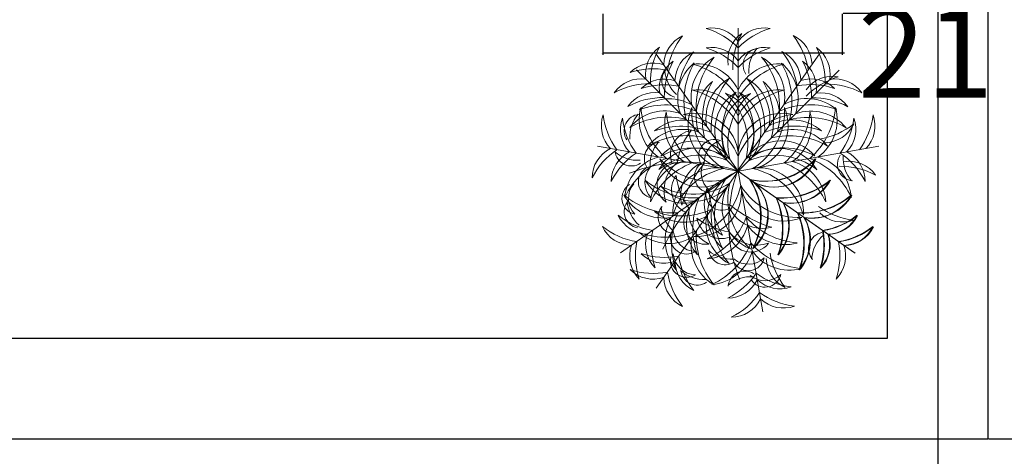
# Model space of a CAD drawing. Units: inches. Extents: x -48 to 50072, y 0 to 21068.
# Tile 33 of 75: x 467 to 555, y 213 to 251. Entities that reach past the tile are written whole.
import ezdxf

# ---------------------------------------------------------------- set-up
doc = ezdxf.new("R2010")
doc.units = ezdxf.units.IN
doc.header["$MEASUREMENT"] = 0
doc.linetypes.add('ACAD_ISO02W100', pattern=[15, 12, -3])
for name, color, linetype, lineweight in [('A-ANNO-DIMS', 2, 'Continuous', 18), ('C-PROP', 7, 'Continuous', 25), ('C-PROP-REF', 32, 'ACAD_ISO02W100', 13), ('L-PLNT', 94, 'Continuous', 13)]:
    doc.layers.add(name, color=color, linetype=linetype, lineweight=lineweight)
doc.styles.get("Standard").update_dxf_attribs({"font": 'arial.ttf'})
doc.dimstyles.get("Standard").update_dxf_attribs({"dimtxt": 8, "dimasz": 0.18, "dimexe": 0.18, "dimexo": 0.0625, "dimgap": 0.09, "dimtad": 0, "dimtih": 1, "dimtoh": 1, "dimdec": 1, "dimzin": 0, "dimdsep": 46, "dimlunit": 4, "dimtxsty": 'Standard', "dimblk": 'ARCHTICK', "dimcen": 0.09, "dimadec": 0, "dimazin": 0, "dimtfac": 1, "dimtdec": 1, "dimtofl": 0, "dimtmove": 0, "dimatfit": 3, "dimldrblk": 'ARCHTICK', "dimfxl": 1, "dimtolj": 1, "dimtzin": 0, "dimarcsym": 0})

# ---------------------------------------------------------------- blocks, each defined once
blk = doc.blocks.new('A$C5D061C3B')
for p, q in [((3.377, 6.679), (3.377, 3.377)), ((1.483, 6.082), (3.377, 3.377)), ((5.259, 6.086), (3.365, 3.381)), ((1.03, 5.716), (3.365, 3.381)), ((5.712, 5.712), (3.377, 3.377)), ((0.125, 3.951), (3.377, 3.377)), ((6.629, 3.951), (3.377, 3.377)), ((0.66, 1.487), (3.365, 3.381)), ((1.483, 0.672), (3.377, 3.377)), ((6.07, 1.487), (3.365, 3.381)), ((3.951, 0.125), (3.377, 3.377)), ((6.082, 1.483), (3.377, 3.377))]:
    blk.add_line(p, q)
for centre, radius, start, end in [((2.763, 5.924), 0.762, 36.29, 99.6243), ((2.145, 5.032), 1.715, 44.0763, 73.3794), ((3.991, 5.924), 0.762, 80.3757, 143.71), ((4.61, 5.032), 1.715, 106.6206, 135.9237), ((2.419, 5.816), 0.762, 115.3757, 178.71), ((3.438, 5.44), 1.715, 141.6206, 170.9237), ((3.901, 5.939), 0.762, 125.3757, 188.71), ((4.969, 5.745), 1.715, 151.6206, 180.9237), ((3.305, 5.444), 1.715, 9.0763, 38.3794), ((4.323, 5.82), 0.762, 1.29, 64.6243), ((1.998, 5.617), 0.762, 125.3757, 188.71), ((3.066, 5.423), 1.715, 151.6206, 180.9237), ((2.763, 5.474), 0.762, 36.29, 99.6243), ((2.145, 4.581), 1.715, 44.0763, 73.3794), ((3.991, 5.474), 0.762, 80.3757, 143.71), ((4.61, 4.581), 1.715, 106.6206, 135.9237), ((3.871, 5.832), 0.38, 94.742, 213.7475), ((4.447, 5.681), 0.826, 139.618, 183.2106), ((4.744, 5.613), 0.762, 351.29, 54.6243), ((3.676, 5.419), 1.715, 359.0763, 28.3794), ((2.317, 5.298), 0.762, 125.3757, 188.71), ((3.385, 5.104), 1.715, 151.6206, 180.9237), ((2.678, 5.447), 0.762, 115.3757, 178.71), ((3.696, 5.07), 1.715, 141.6206, 170.9237), ((3.344, 5.089), 1.056, 119.6063, 189.7511), ((4.177, 4.869), 1.77, 139.9634, 183.6288), ((3.398, 5.094), 1.056, 350.2489, 60.3937), ((2.565, 4.873), 1.77, 356.3712, 40.0366), ((4.064, 5.451), 0.762, 1.29, 64.6243), ((3.046, 5.075), 1.715, 9.0763, 38.3794), ((1.413, 5.111), 0.762, 71.29, 134.6243), ((1.419, 4.026), 1.715, 79.0763, 108.3794), ((1.991, 5.462), 0.38, 139.742, 258.7475), ((2.505, 5.763), 0.826, 184.618, 228.2106), ((3.035, 5.062), 1.056, 129.6063, 199.7511), ((3.894, 4.989), 1.77, 149.9634, 193.6288), ((2.422, 4.799), 1.056, 25.2489, 95.3937), ((1.866, 4.14), 1.77, 31.3712, 75.0366), ((4.332, 4.799), 1.056, 84.6063, 154.7511), ((4.888, 4.14), 1.77, 104.9634, 148.6288), ((2.848, 4.985), 1.77, 346.3712, 30.0366), ((3.707, 5.058), 1.056, 340.2489, 50.3937), ((3.357, 5.1), 1.715, 359.0763, 28.3794), ((4.425, 5.294), 0.762, 351.29, 54.6243), ((1.13, 4.748), 0.762, 81.29, 144.6243), ((1.671, 4.742), 0.762, 71.29, 134.6243), ((3.688, 4.597), 1.056, 119.6063, 189.7511), ((4.522, 4.377), 1.77, 139.9634, 183.6288), ((2.221, 4.381), 1.77, 356.3712, 40.0366), ((3.054, 4.602), 1.056, 350.2489, 60.3937), ((5.071, 4.746), 0.762, 45.3757, 108.71), ((5.564, 4.807), 0.762, 80.3757, 143.71), ((6.182, 3.914), 1.715, 106.6206, 135.9237), ((5.613, 4.744), 0.762, 35.3757, 98.71), ((1.324, 3.68), 1.715, 89.0763, 118.3794), ((1.677, 3.657), 1.715, 79.0763, 108.3794), ((2.422, 4.198), 1.056, 25.2489, 95.3937), ((1.866, 3.54), 1.77, 31.3712, 75.0366), ((3.46, 4.637), 1.056, 129.6063, 199.7511), ((4.319, 4.565), 1.77, 149.9634, 193.6288), ((4.332, 4.198), 1.056, 84.6063, 154.7511), ((4.888, 3.54), 1.77, 104.9634, 148.6288), ((3.283, 4.633), 1.056, 340.2489, 50.3937), ((2.424, 4.56), 1.77, 346.3712, 30.0366), ((5.065, 3.661), 1.715, 71.6206, 100.9237), ((5.419, 3.676), 1.715, 61.6206, 90.9237), ((1.448, 4.43), 0.762, 81.29, 144.6243), ((1.642, 3.362), 1.715, 89.0763, 118.3794), ((1.78, 3.994), 1.056, 60.2489, 130.3937), ((3.868, 4.321), 1.029, 121.3654, 221.5741), ((4.556, 4.237), 1.557, 141.8122, 203.3335), ((4.035, 4.215), 1.029, 111.3654, 211.5741), ((2.707, 4.219), 1.029, 328.4259, 68.6346), ((2.044, 4.017), 1.557, 346.6665, 48.1878), ((4.698, 4.013), 1.557, 131.8122, 193.3335), ((2.187, 4.233), 1.557, 336.6665, 38.1878), ((2.875, 4.316), 1.029, 318.4259, 58.6346), ((4.963, 3.998), 1.056, 49.6063, 119.7511), ((5.1, 3.357), 1.715, 61.6206, 90.9237), ((5.294, 4.425), 0.762, 35.3757, 98.71), ((2.143, 4.564), 1.056, 164.6063, 234.7511), ((1.702, 3.136), 1.77, 66.3712, 110.0366), ((2.888, 4.998), 1.77, 184.9634, 228.6288), ((3.25, 4.435), 1.029, 156.3654, 256.5741), ((3.862, 4.761), 1.557, 176.8122, 238.3335), ((2.893, 4.761), 1.557, 301.6665, 3.1878), ((3.504, 4.435), 1.029, 283.4259, 23.6346), ((5.04, 3.14), 1.77, 69.9634, 113.6288), ((3.866, 4.998), 1.77, 311.3712, 355.0366), ((4.611, 4.564), 1.056, 305.2489, 15.3937), ((0.975, 4.424), 0.762, 160.3757, 223.71), ((1.962, 4.878), 1.715, 186.6206, 215.9237), ((1.419, 4.346), 0.762, 160.3757, 223.71), ((2.405, 4.8), 1.715, 186.6206, 215.9237), ((1.12, 4.31), 0.38, 94.742, 213.7475), ((1.696, 4.159), 0.826, 139.618, 183.2106), ((1.685, 3.712), 1.056, 70.2489, 140.3937), ((1.757, 2.853), 1.77, 76.3712, 120.0366), ((2.124, 3.502), 1.056, 60.2489, 130.3937), ((2.734, 4.46), 1.056, 164.6063, 234.7511), ((3.48, 4.893), 1.77, 184.9634, 228.6288), ((2.358, 3.686), 1.029, 3.4259, 103.6346), ((1.93, 3.14), 1.557, 21.6665, 83.1878), ((4.397, 3.686), 1.029, 76.3654, 176.5741), ((4.824, 3.14), 1.557, 96.8122, 158.3335), ((4.618, 3.506), 1.056, 49.6063, 119.7511), ((3.275, 4.893), 1.77, 311.3712, 355.0366), ((4.985, 2.848), 1.77, 59.9634, 103.6288), ((4.02, 4.46), 1.056, 305.2489, 15.3937), ((5.058, 3.707), 1.056, 39.6063, 109.7511), ((4.349, 4.8), 1.715, 324.0763, 353.3794), ((5.335, 4.346), 0.762, 316.29, 19.6243), ((4.793, 4.878), 1.715, 324.0763, 353.3794), ((5.779, 4.424), 0.762, 316.29, 19.6243), ((2.109, 3.287), 1.056, 70.2489, 140.3937), ((2.046, 2.644), 1.77, 66.3712, 110.0366), ((4.696, 2.648), 1.77, 69.9634, 113.6288), ((4.633, 3.283), 1.056, 39.6063, 109.7511), ((4.988, 5.812), 1.715, 279.0763, 308.3794), ((5.365, 4.794), 0.762, 271.29, 334.6243), ((2.182, 2.428), 1.77, 76.3712, 120.0366), ((2.387, 3.752), 0.574, 99.9865, 199.4034), ((3.599, 3.314), 1.651, 142.5759, 170.8942), ((2.84, 3.739), 0.372, 69.2257, 210.1279), ((4.56, 2.424), 1.77, 59.9634, 103.6288), ((0.762, 3.214), 0.762, 116.29, 179.6243), ((1.534, 2.451), 1.715, 124.0763, 153.3794), ((1.588, 3.666), 0.38, 94.742, 213.7475), ((2.165, 3.515), 0.826, 139.618, 183.2106), ((2.426, 2.879), 1.029, 48.4259, 148.6346), ((2.365, 3.045), 1.029, 38.4259, 138.6346), ((2.328, 2.353), 1.557, 56.6665, 118.1878), ((3.109, 3.59), 0.515, 105.4398, 183.6694), ((4.414, 2.358), 1.557, 61.8122, 123.3335), ((4.377, 3.05), 1.029, 41.3654, 141.5741), ((4.316, 2.875), 1.029, 31.3654, 131.5741), ((1.206, 3.136), 0.762, 116.29, 179.6243), ((1.977, 2.373), 1.715, 124.0763, 153.3794), ((1.062, 4.452), 0.826, 229.618, 273.2106), ((0.91, 3.875), 0.38, 184.742, 303.7475), ((1.811, 2.684), 1.056, 105.2489, 175.3937), ((2.363, 2.022), 1.77, 111.3712, 155.0366), ((2.51, 2.191), 1.557, 66.6665, 128.1878), ((2.729, 4.702), 1.557, 221.8122, 283.3335), ((2.527, 4.039), 1.029, 201.3654, 301.5741), ((4.233, 2.187), 1.557, 51.8122, 113.3335), ((4.001, 4.702), 1.557, 256.6665, 318.1878), ((4.013, 4.698), 1.557, 256.6665, 318.1878), ((4.203, 4.039), 1.029, 238.4259, 338.6346), ((4.215, 4.035), 1.029, 238.4259, 338.6346), ((4.391, 2.022), 1.77, 24.9634, 68.6288), ((4.943, 2.684), 1.056, 4.6063, 74.7511), ((6.053, 3.533), 0.38, 146.2525, 265.258), ((4.777, 2.373), 1.715, 26.6206, 55.9237), ((6.629, 3.684), 0.826, 176.7894, 220.382), ((5.549, 3.136), 0.762, 0.3757, 63.71), ((2.185, 0.015), 3.567, 70.4772, 111.6585), ((1.447, 3.129), 0.376, 122.0577, 257.8533), ((1.751, 3.126), 0.529, 140.1845, 223.654), ((2.403, 2.58), 1.056, 105.2489, 175.3937), ((2.955, 1.917), 1.77, 111.3712, 155.0366), ((2.007, 3.071), 0.506, 93.8744, 233.9763), ((2.489, 2.932), 0.825, 128.7536, 199.097), ((2.896, 2.427), 1.029, 83.4259, 183.6346), ((3.359, 1.911), 1.557, 101.6665, 163.1878), ((2.903, 2.8), 0.855, 116.4477, 194.3672), ((4.744, 1.779), 2.789, 140.4007, 163.139), ((2.741, 3.253), 0.372, 114.2257, 255.1279), ((3.037, 3.338), 0.515, 150.4398, 228.6694), ((3.395, 1.911), 1.557, 16.8122, 78.3335), ((3.858, 2.427), 1.029, 356.3654, 96.5741), ((3.799, 1.917), 1.77, 24.9634, 68.6288), ((4.352, 2.58), 1.056, 4.6063, 74.7511), ((5.741, 1.774), 1.715, 61.6206, 90.9237), ((5.935, 2.842), 0.762, 35.3757, 98.71), ((4.912, 0.157), 3.567, 115.4772, 156.6585), ((2.412, 2.943), 0.574, 144.9865, 244.4034), ((3.578, 3.49), 1.651, 187.5759, 215.8942), ((4.389, 2.332), 1.557, 146.6665, 208.1878), ((6.727, 2.189), 3.567, 160.4772, 201.6585), ((2.341, 2.332), 1.557, 331.8122, 33.3335), ((1.067, 2.749), 0.376, 122.0577, 257.8533), ((1.37, 2.745), 0.529, 140.1845, 223.654), ((2.145, 3.693), 1.056, 209.6063, 279.7511), ((2.365, 4.526), 1.77, 229.9634, 273.6288), ((2.328, 4.401), 1.557, 241.8122, 303.3335), ((2.365, 3.709), 1.029, 221.3654, 321.5741), ((1.911, 3.359), 1.557, 286.8122, 348.3335), ((2.427, 2.896), 1.029, 266.3654, 6.5741), ((3.003, 2.844), 0.372, 159.2257, 300.1279), ((3.152, 3.113), 0.515, 195.4398, 273.6694), ((3.697, 2.369), 1.029, 128.4259, 228.6346), ((4.035, 2.539), 1.029, 148.4259, 248.6346), ((4.698, 2.741), 1.557, 166.6665, 228.1878), ((4.435, 3.25), 1.029, 193.4259, 293.6346), ((4.761, 3.862), 1.557, 211.6665, 273.1878), ((2.353, 2.328), 1.557, 331.8122, 33.3335), ((3.033, 2.369), 1.029, 311.3654, 51.5741), ((3.045, 2.365), 1.029, 311.3654, 51.5741), ((4.365, 4.526), 1.77, 266.3712, 310.0366), ((4.377, 4.522), 1.77, 266.3712, 310.0366), ((4.585, 3.693), 1.056, 260.2489, 330.3937), ((4.597, 3.688), 1.056, 260.2489, 330.3937), ((1.873, 4.181), 1.77, 229.9634, 273.6288), ((1.653, 3.348), 1.056, 209.6063, 279.7511), ((4.099, 2.051), 1.77, 156.3712, 200.0366), ((3.45, 2.634), 0.855, 161.4477, 239.3672), ((5.474, 3.214), 2.789, 185.4007, 208.139), ((2.632, 2.051), 1.77, 339.9634, 23.6288), ((2.644, 2.046), 1.77, 339.9634, 23.6288), ((4.857, 4.181), 1.77, 266.3712, 310.0366), ((4.869, 4.177), 1.77, 266.3712, 310.0366), ((5.077, 3.348), 1.056, 260.2489, 330.3937), ((5.089, 3.344), 1.056, 260.2489, 330.3937), ((1.122, 2.441), 0.38, 139.742, 258.7475), ((1.636, 2.741), 0.826, 184.618, 228.2106), ((1.908, 2.317), 0.38, 139.742, 258.7475), ((2.422, 2.617), 0.826, 184.618, 228.2106), ((2.624, 2.192), 0.506, 138.8744, 278.9763), ((3.24, 2.128), 1.056, 150.2489, 220.3937), ((3.064, 2.435), 0.825, 173.7536, 244.097), ((3.942, 2.908), 0.855, 206.4477, 284.3672), ((4.963, 4.749), 2.789, 230.4007, 253.139), ((3.49, 2.128), 1.056, 319.6063, 29.7511), ((3.502, 2.124), 1.056, 319.6063, 29.7511), ((6.244, 3.948), 1.715, 234.0763, 263.3794), ((1.672, 3.7), 1.715, 231.6206, 260.9237), ((1.295, 2.682), 0.762, 205.3757, 268.71), ((2.046, 4.111), 1.77, 249.9634, 293.6288), ((2.124, 3.252), 1.056, 229.6063, 299.7511), ((2.748, 1.784), 1.056, 150.2489, 220.3937), ((3.607, 1.706), 1.77, 156.3712, 200.0366), ((3.428, 3.603), 1.651, 232.5759, 260.8942), ((2.99, 2.391), 0.574, 189.9865, 289.4034), ((3.688, 2.157), 1.056, 170.2489, 240.3937), ((1.917, 2.955), 1.77, 294.9634, 338.6288), ((4.522, 2.378), 1.77, 176.3712, 220.0366), ((4.893, 3.48), 1.77, 221.3712, 265.0366), ((3.124, 1.706), 1.77, 339.9634, 23.6288), ((3.136, 1.702), 1.77, 339.9634, 23.6288), ((3.982, 1.784), 1.056, 319.6063, 29.7511), ((3.994, 1.78), 1.056, 319.6063, 29.7511), ((5.79, 2.962), 0.762, 226.29, 289.6243), ((5.058, 3.7), 1.715, 279.0763, 308.3794), ((5.07, 3.696), 1.715, 279.0763, 308.3794), ((5.435, 2.682), 0.762, 271.29, 334.6243), ((5.447, 2.678), 0.762, 271.29, 334.6243), ((0.926, 2.424), 0.762, 205.3757, 268.71), ((1.303, 3.442), 1.715, 231.6206, 260.9237), ((2.58, 2.403), 1.056, 274.6063, 344.7511), ((4.46, 2.734), 1.056, 215.2489, 285.3937), ((5.427, 3.442), 1.715, 279.0763, 308.3794), ((5.44, 3.438), 1.715, 279.0763, 308.3794), ((5.804, 2.424), 0.762, 271.29, 334.6243), ((5.816, 2.419), 0.762, 271.29, 334.6243), ((1.702, 3.619), 1.77, 249.9634, 293.6288), ((1.78, 2.76), 1.056, 229.6063, 299.7511), ((2, 1.676), 0.762, 161.29, 224.6243), ((3.086, 1.681), 1.715, 169.0763, 198.3794), ((2.188, 1.837), 0.376, 167.0577, 302.8533), ((2.405, 2.049), 0.529, 185.1845, 268.654), ((3.344, 1.665), 1.056, 170.2489, 240.3937), ((4.177, 1.886), 1.77, 176.3712, 220.0366), ((3.81, 2.493), 0.825, 218.7536, 289.097), ((3.671, 2.011), 0.506, 183.8744, 323.9763), ((5.385, 1.584), 0.38, 101.2525, 220.258), ((5.899, 1.283), 0.826, 131.7894, 175.382), ((3.645, 1.681), 1.715, 341.6206, 10.9237), ((4.73, 1.676), 0.762, 315.3757, 18.71), ((3.657, 1.677), 1.715, 341.6206, 10.9237), ((4.742, 1.671), 0.762, 315.3757, 18.71), ((1.631, 1.417), 0.762, 161.29, 224.6243), ((2.717, 1.423), 1.715, 169.0763, 198.3794), ((2.022, 2.363), 1.77, 294.9634, 338.6288), ((4.998, 2.888), 1.77, 221.3712, 265.0366), ((4.014, 1.423), 1.715, 341.6206, 10.9237), ((5.099, 1.417), 0.762, 315.3757, 18.71), ((1.671, 2.012), 0.762, 225.3757, 288.71), ((1.677, 3.098), 1.715, 251.6206, 280.9237), ((2.188, 1.299), 0.376, 167.0577, 302.8533), ((2.405, 1.511), 0.529, 185.1845, 268.654), ((3.696, 1.684), 1.715, 189.0763, 218.3794), ((3.227, 2.169), 0.826, 229.618, 273.2106), ((3.076, 1.593), 0.38, 184.742, 303.7475), ((2.684, 1.811), 1.056, 274.6063, 344.7511), ((3.616, 1.755), 0.529, 230.1845, 313.654), ((3.613, 1.452), 0.376, 212.0577, 347.8533), ((4.564, 2.143), 1.056, 215.2489, 285.3937), ((5.808, 1.754), 1.715, 189.0763, 218.3794), ((2.678, 1.307), 0.762, 181.29, 244.6243), ((4.79, 1.377), 0.762, 181.29, 244.6243), ((1.419, 2.729), 1.715, 251.6206, 280.9237), ((1.413, 1.643), 0.762, 225.3757, 288.71), ((2.419, 0.938), 0.762, 181.29, 244.6243), ((3.438, 1.315), 1.715, 189.0763, 218.3794), ((2.583, 1.701), 0.826, 229.618, 273.2106), ((2.432, 1.124), 0.38, 184.742, 303.7475), ((2.373, 1.977), 1.715, 296.6206, 325.9237), ((3.68, 0.113), 0.826, 86.7894, 130.382), ((3.528, 0.69), 0.38, 56.2525, 175.258), ((3.997, 1.374), 0.529, 230.1845, 313.654), ((3.994, 1.071), 0.376, 212.0577, 347.8533), ((4.8, 2.405), 1.715, 234.0763, 263.3794), ((3.136, 1.206), 0.762, 270.3757, 333.71), ((4.346, 1.419), 0.762, 226.29, 289.6243), ((2.451, 1.534), 1.715, 296.6206, 325.9237), ((4.878, 1.962), 1.715, 234.0763, 263.3794), ((3.214, 0.762), 0.762, 270.3757, 333.71), ((4.424, 0.975), 0.762, 226.29, 289.6243)]:
    blk.add_arc(centre, radius, start, end)
blk = doc.blocks.new('_ArchTick')
at = {"color": 0, "linetype": 'ByBlock', "const_width": 0.15}
blk.add_lwpolyline([(-0.5, -0.5), (0.5, 0.5)], dxfattribs=at)
blk = doc.blocks.new('*D54')
at = {"layer": 'A-ANNO-DIMS', "color": 0, "lineweight": -2, "transparency": 16777216}
for p, q in [((540.551, 275.597), (544.198, 275.597)), ((544.018, 275.597), (544.018, 268.06)), ((544.018, 252.07), (544.018, 259.607)), ((540.551, 252.07), (544.198, 252.07))]:
    blk.add_line(p, q, dxfattribs=at)
at = {"layer": 'Defpoints', "color": 0, "transparency": 16777216}
for p in [(540.489, 275.597), (544.018, 275.597), (540.489, 252.07)]:
    blk.add_point(p, dxfattribs=at)
at = {"layer": 'A-ANNO-DIMS', "color": 0, "lineweight": -2, "transparency": 16777216, "xscale": 0.18, "yscale": 0.18, "zscale": 0.18}
for p, rotation in [((544.018, 275.597), 90), ((544.018, 252.07), 270)]:
    blk.add_blockref('_ArchTick', p, dxfattribs=dict(at, rotation=rotation))
at = {"layer": 'A-ANNO-DIMS', "color": 0, "transparency": 16777216, "insert": (544.018, 263.834), "char_height": 8, "attachment_point": 5}
blk.add_mtext('\\A1;SHRUB B 24 TYP.', dxfattribs=at)
blk = doc.blocks.new('*D55')
at = {"layer": 'A-ANNO-DIMS', "color": 0, "lineweight": -2, "transparency": 16777216}
for p, q in [((519.098, 252.008), (519.098, 248.361)), ((540.489, 252.008), (540.489, 248.361)), ((519.098, 248.541), (540.489, 248.541)), ((540.489, 248.541), (540.669, 248.541))]:
    blk.add_line(p, q, dxfattribs=at)
at = {"layer": 'Defpoints', "color": 0, "transparency": 16777216}
for p in [(519.098, 252.07), (540.489, 252.07), (540.489, 248.541)]:
    blk.add_point(p, dxfattribs=at)
at = {"layer": 'A-ANNO-DIMS', "color": 0, "lineweight": -2, "transparency": 16777216, "xscale": 0.18, "yscale": 0.18, "zscale": 0.18, "rotation": 180}
blk.add_blockref('_ArchTick', (519.098, 248.541), dxfattribs=at)
at = {"layer": 'A-ANNO-DIMS', "color": 0, "lineweight": -2, "transparency": 16777216, "xscale": 0.18, "yscale": 0.18, "zscale": 0.18}
blk.add_blockref('_ArchTick', (540.489, 248.541), dxfattribs=at)
at = {"layer": 'A-ANNO-DIMS', "color": 0, "transparency": 16777216, "insert": (560.298, 248.541), "char_height": 8, "attachment_point": 5}
blk.add_mtext('\\A1;21 TYP.', dxfattribs=at)
blk = doc.blocks.new('*D115')
at = {"layer": 'A-ANNO-DIMS', "color": 0, "lineweight": -2, "transparency": 16777216}
for p, q in [((549.08, 451.075), (601.647, 451.075)), ((601.467, 451.075), (601.467, 336.752)), ((601.467, 214.075), (601.467, 328.397)), ((553.58, 214.075), (601.647, 214.075))]:
    blk.add_line(p, q, dxfattribs=at)
at = {"layer": 'Defpoints', "color": 0, "transparency": 16777216}
for p in [(549.017, 451.075), (601.467, 451.075), (553.517, 214.075)]:
    blk.add_point(p, dxfattribs=at)
at = {"layer": 'A-ANNO-DIMS', "color": 0, "lineweight": -2, "transparency": 16777216, "xscale": 0.18, "yscale": 0.18, "zscale": 0.18}
for p, rotation in [((601.467, 451.075), 90), ((601.467, 214.075), 270)]:
    blk.add_blockref('_ArchTick', p, dxfattribs=dict(at, rotation=rotation))
at = {"layer": 'A-ANNO-DIMS', "color": 0, "transparency": 16777216, "insert": (601.467, 332.575), "char_height": 8, "attachment_point": 5}
blk.add_mtext('\\A1;237', dxfattribs=at)
blk = doc.blocks.new('*D119')
at = {"layer": 'A-ANNO-DIMS', "color": 0, "lineweight": -2, "transparency": 16777216}
for p, q in [((463.517, 451.012), (463.517, 165.945)), ((549.017, 451.012), (549.017, 165.945)), ((463.517, 166.125), (495.752, 166.125)), ((549.017, 166.125), (516.783, 166.125))]:
    blk.add_line(p, q, dxfattribs=at)
at = {"layer": 'Defpoints', "color": 0, "transparency": 16777216}
for p in [(463.517, 451.075), (549.017, 451.075), (549.017, 166.125)]:
    blk.add_point(p, dxfattribs=at)
at = {"layer": 'A-ANNO-DIMS', "color": 0, "lineweight": -2, "transparency": 16777216, "xscale": 0.18, "yscale": 0.18, "zscale": 0.18, "rotation": 180}
blk.add_blockref('_ArchTick', (463.517, 166.125), dxfattribs=at)
at = {"layer": 'A-ANNO-DIMS', "color": 0, "lineweight": -2, "transparency": 16777216, "xscale": 0.18, "yscale": 0.18, "zscale": 0.18}
blk.add_blockref('_ArchTick', (549.017, 166.125), dxfattribs=at)
at = {"layer": 'A-ANNO-DIMS', "color": 0, "transparency": 16777216, "insert": (506.267, 166.125), "char_height": 8, "attachment_point": 5}
blk.add_mtext('\\A1;85.5', dxfattribs=at)

msp = doc.modelspace()

# ---------------------------------------------------------------- linework, layer by layer
at = {"layer": 'C-PROP'}
for p, q in [((553.517, 214.075), (553.517, 1170.775)), ((544.517, 223.075), (544.517, 488.775)), ((210.389, 223.075), (544.517, 223.075)), ((210.389, 214.075), (553.517, 214.075))]:
    msp.add_line(p, q, dxfattribs=at)
at = {"layer": 'C-PROP-REF'}
msp.add_line((549.017, 214.075), (549.017, 1166.275), dxfattribs=at)

# ---------------------------------------------------------------- block references
at = {"layer": 'L-PLNT', "xscale": 3.862191520948588, "yscale": 3.862191520948588, "zscale": 3.862191520948588}
msp.add_blockref('A$C5D061C3B', (518.144, 224.93), dxfattribs=at)

# ---------------------------------------------------------------- dimensions: what is measured, and where the dimension line sits
at = {"layer": 'A-ANNO-DIMS'}
dim = msp.add_linear_dim(base=(549.017, 166.125), p1=(463.517, 451.075), p2=(549.017, 451.075), dimstyle='Standard', override={"dimdec": 1, "dimlfac": 1, "dimrnd": 0, "dimzin": 0, "dimdsep": 46, "dimlunit": 2}, dxfattribs=at)
dim.commit()
dim.dimension.update_dxf_attribs({"geometry": '*D119', "text_midpoint": (506.267, 166.125)})
dim = msp.add_linear_dim(base=(601.467, 451.075), p1=(553.517, 214.075), p2=(549.017, 451.075), angle=90, dimstyle='Standard', override={"dimdec": 0, "dimlfac": 1, "dimrnd": 0, "dimzin": 0, "dimdsep": 46, "dimlunit": 2}, dxfattribs=at)
dim.commit()
dim.dimension.update_dxf_attribs({"geometry": '*D115', "text_midpoint": (601.467, 332.575)})
dim = msp.add_linear_dim(base=(544.018, 275.597), p1=(540.489, 252.07), p2=(540.489, 275.597), angle=90, text='SHRUB B <> TYP.', dimstyle='Standard', override={"dimdec": 0, "dimlfac": 1, "dimrnd": 0, "dimzin": 0, "dimdsep": 46, "dimlunit": 2}, dxfattribs=at)
dim.commit()
dim.dimension.update_dxf_attribs({"geometry": '*D54', "text_midpoint": (544.018, 263.834)})
dim = msp.add_linear_dim(base=(540.489, 248.541), p1=(519.098, 252.07), p2=(540.489, 252.07), text='<> TYP.', dimstyle='Standard', override={"dimdec": 0, "dimlfac": 1, "dimrnd": 0, "dimzin": 0, "dimdsep": 46, "dimlunit": 2}, dxfattribs=at)
dim.commit()
dim.dimension.update_dxf_attribs({"geometry": '*D55', "text_midpoint": (560.298, 248.541)})

doc.saveas('drawing.dxf')
